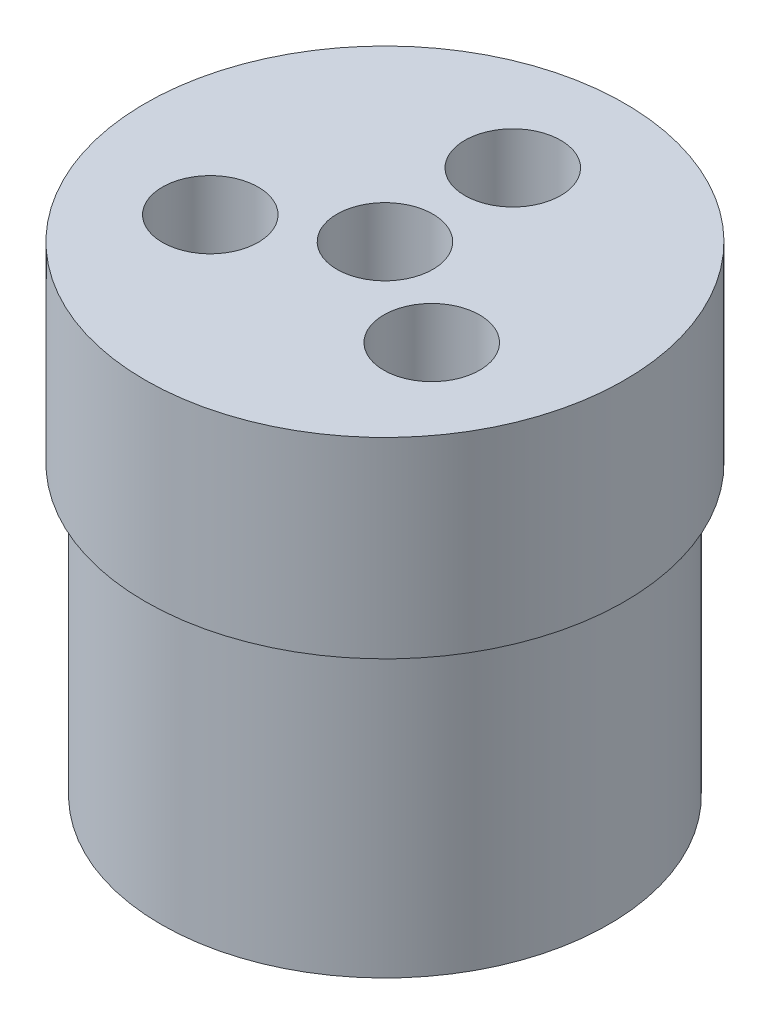
SolidWorks part; units mm, degrees
material "Plain Carbon Steel"
ref_plane "Front Plane" through (0, 0, 0) normal (0, 0, 1) x (1, 0, 0)
ref_plane "Top Plane" through (0, 0, 0) normal (0, 1, 0) x (1, 0, 0)
ref_plane "Right Plane" through (0, 0, 0) normal (1, 0, 0) x (0, 0, -1)
sketch "Upper Body Profile Ø30" plane through (0, 0, 0) normal (0, 1, 0) x (1, 0, 0)
  circle A0 centre (0, 0) radius 15
  dimension "D1" = 30
extrude "Upper Body Ø30x12" add sketch "Upper Body Profile Ø30" along normal blind 12
sketch "Lower Body Profile Ø28" plane through (0, 0, 0) normal (0, -1, 0) x (1, 0, 0)
  circle A0 centre (0, 0) radius 14
  dimension "D1" = 28
extrude "Lower Body Ø28x18" add sketch "Lower Body Profile Ø28" along normal blind 18
sketch "Offset Holes Profile 3xØ6" plane through (0, 12, 0) normal (0, 1, 0) x (1, 0, 0)
  circle A0 centre (0, 0) radius 8 construction
  circle A1 centre (0, 8) radius 3
  circle A2 centre (6.9282, -4) radius 3
  circle A3 centre (-6.9282, -4) radius 3
  dimension "D1" = 16
  dimension "D2" = 6
  dimension "D4" = 6.9282
  dimension "D5" = 4
  dimension "D3" = 3
extrude "Offset Through Holes 3xØ6" cut sketch "Offset Holes Profile 3xØ6" against normal blind 44
sketch "Center Hole Profile Ø6" plane through (0, 12, 0) normal (0, 1, 0) x (1, 0, 0)
  circle A0 centre (0, 0) radius 3
  dimension "D1" = 6
extrude "Center Through Hole Ø6" cut sketch "Center Hole Profile Ø6" against normal blind 44
